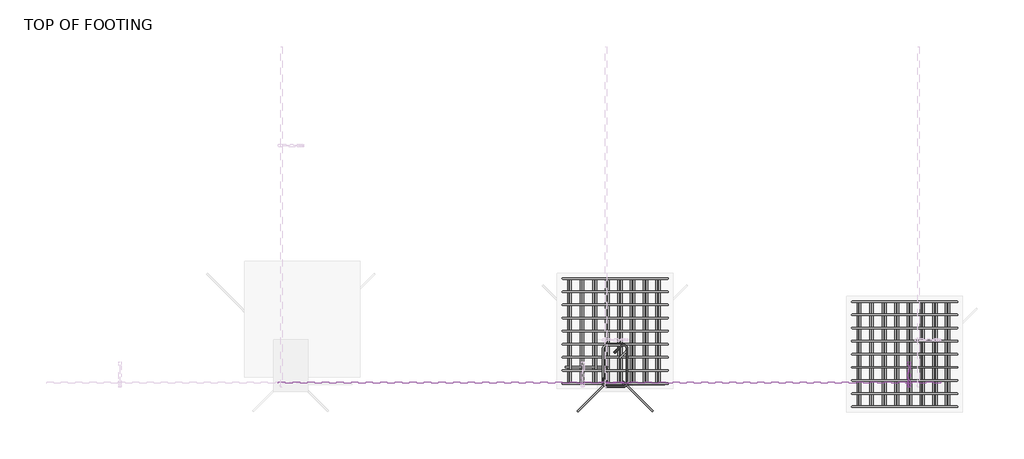
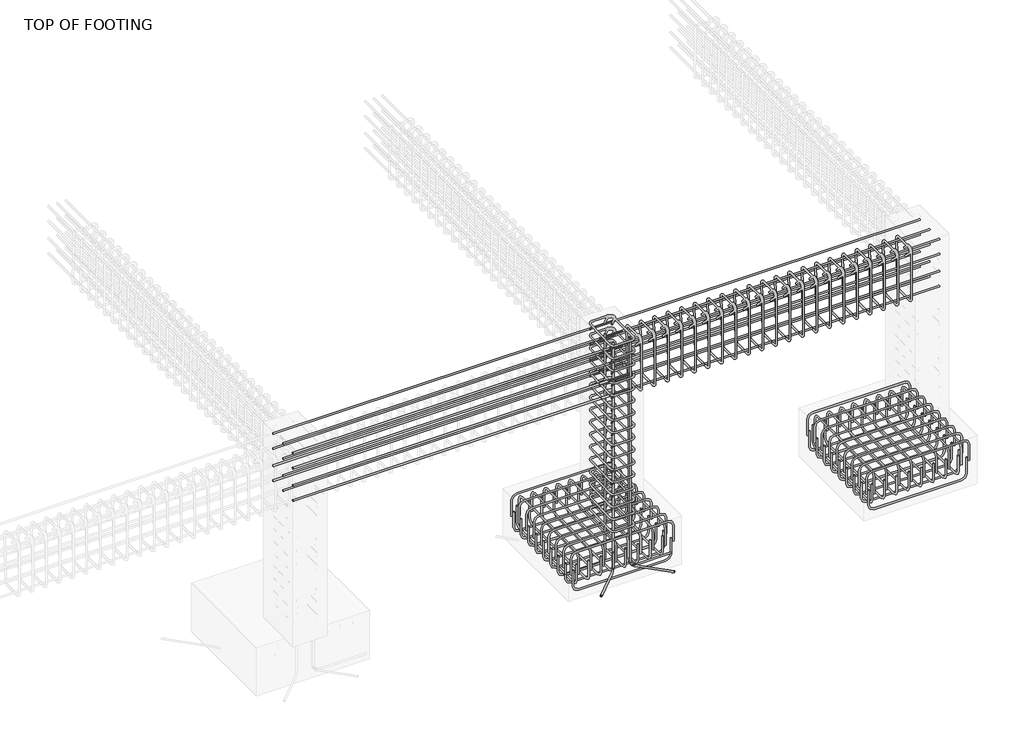
# One storey, part 3 of 14: 22 reinforcing bars.
"""IFC4 building model written with IfcOpenShell, lengths in millimetres."""

from ifc_helpers import new_model, si_unit, point, frame, origin, place, context, project, spatial, polyline, circle_curve, trimmed, segment, composite_curve, source, transform, mapped, element, save
from ifc_brep_helpers import swept_disk

model = new_model("IFC4")

# Units and contexts
model_context = context("Model", 3, world=origin())
ifc_project = project(units=[si_unit("LENGTHUNIT", "METRE", prefix="MILLI")], contexts=[model_context])

# Site, building, storey
site = spatial("IfcSite", under=ifc_project)
building = spatial("IfcBuilding", under=site)
storey = spatial("IfcBuildingStorey", under=building, Name="TOP OF FOOTING", Elevation=-1828.8)

# Reinforcing bars
placement = place(None, origin())
reinforcing_bar_shape = source(origin(), model_context, "Body", "SolidModel", [
    swept_disk(composite_curve([segment(polyline([(4972.542187, 217.7803241, -2035.6107622), (4972.542187, 217.7803241, -2182.9107622)]), True, "CONTINUOUS"), segment(trimmed(circle_curve(frame((4926.192187, 217.7803241, -2182.9107622), z_axis=(0.0, 1.0, 0.0), x_axis=(46.350000000000364, 0.0, 0.0)), 46.35), [point((4972.542187, 217.7803241, -2182.9107622))], [point((4926.192187, 217.7803241, -2229.2607622))], True, "CARTESIAN"), True, "CONTINUOUS"), segment(polyline([(4926.192187, 217.7803241, -2229.2607622), (4153.5617984, 217.7803241, -2229.2607622)]), True, "CONTINUOUS"), segment(trimmed(circle_curve(frame((4153.5617984, 217.7803241, -2182.9107622), z_axis=(0.0, 1.0, 0.0), x_axis=(0.0, 0.0, -46.34999999999991)), 46.35), [point((4153.5617984, 217.7803241, -2229.2607622))], [point((4107.2117984, 217.7803241, -2182.9107622))], True, "CARTESIAN"), True, "CONTINUOUS"), segment(polyline([(4107.2117984, 217.7803241, -2182.9107622), (4107.2117984, 217.7803241, -2035.6107622)]), True, "CONTINUOUS")], self_intersect=False), 6.35),
])
element("IfcReinforcingBar", 1, at=placement, inside=storey, context=model_context, shape_type="MappedRepresentation", body=[
    mapped(reinforcing_bar_shape, transform((0.0, 0.0, 0.0), x_axis=(1.0, 0.0, 0.0), y_axis=(0.0, 1.0, 0.0), z_axis=(0.0, 0.0, 1.0))),
    mapped(reinforcing_bar_shape, transform((0.0, -113.4125, 0.0), x_axis=(1.0, 0.0, 0.0), y_axis=(0.0, 1.0, 0.0), z_axis=(0.0, 0.0, 1.0))),
    mapped(reinforcing_bar_shape, transform((0.0, -226.825, 0.0), x_axis=(1.0, 0.0, 0.0), y_axis=(0.0, 1.0, 0.0), z_axis=(0.0, 0.0, 1.0))),
    mapped(reinforcing_bar_shape, transform((0.0, -340.2375, 0.0), x_axis=(1.0, 0.0, 0.0), y_axis=(0.0, 1.0, 0.0), z_axis=(0.0, 0.0, 1.0))),
    mapped(reinforcing_bar_shape, transform((0.0, -453.65, 0.0), x_axis=(1.0, 0.0, 0.0), y_axis=(0.0, 1.0, 0.0), z_axis=(0.0, 0.0, 1.0))),
    mapped(reinforcing_bar_shape, transform((0.0, -567.0625, 0.0), x_axis=(1.0, 0.0, 0.0), y_axis=(0.0, 1.0, 0.0), z_axis=(0.0, 0.0, 1.0))),
    mapped(reinforcing_bar_shape, transform((0.0, -680.475, 0.0), x_axis=(1.0, 0.0, 0.0), y_axis=(0.0, 1.0, 0.0), z_axis=(0.0, 0.0, 1.0))),
    mapped(reinforcing_bar_shape, transform((0.0, -793.8875, 0.0), x_axis=(1.0, 0.0, 0.0), y_axis=(0.0, 1.0, 0.0), z_axis=(0.0, 0.0, 1.0))),
    mapped(reinforcing_bar_shape, transform((0.0, -907.3, 0.0), x_axis=(1.0, 0.0, 0.0), y_axis=(0.0, 1.0, 0.0), z_axis=(0.0, 0.0, 1.0))),
])
reinforcing_bar_2_shape = source(origin(), model_context, "Body", "SolidModel", [
    swept_disk(composite_curve([segment(polyline([(4088.9966213, 217.7803241, -2068.991024), (4088.9966213, 217.7803241, -1921.691024)]), True, "CONTINUOUS"), segment(trimmed(circle_curve(frame((4135.3466213, 217.7803241, -1921.691024), z_axis=(0.0, 1.0, 0.0), x_axis=(-46.350000000000364, 0.0, 0.0)), 46.35), [point((4088.9966213, 217.7803241, -1921.691024))], [point((4135.3466213, 217.7803241, -1875.341024))], True, "CARTESIAN"), True, "CONTINUOUS"), segment(polyline([(4135.3466213, 217.7803241, -1875.341024), (4949.9466213, 217.7803241, -1875.341024)]), True, "CONTINUOUS"), segment(trimmed(circle_curve(frame((4949.9466213, 217.7803241, -1921.691024), z_axis=(0.0, 1.0, 0.0), x_axis=(0.0, 0.0, 46.34999999999991)), 46.35), [point((4949.9466213, 217.7803241, -1875.341024))], [point((4996.2966213, 217.7803241, -1921.691024))], True, "CARTESIAN"), True, "CONTINUOUS"), segment(polyline([(4996.2966213, 217.7803241, -1921.691024), (4996.2966213, 217.7803241, -2068.991024)]), True, "CONTINUOUS")], self_intersect=False), 6.35),
])
element("IfcReinforcingBar", 2, at=placement, inside=storey, context=model_context, shape_type="MappedRepresentation", body=[
    mapped(reinforcing_bar_2_shape, transform((0.0, 0.0, 0.0), x_axis=(1.0, 0.0, 0.0), y_axis=(0.0, 1.0, 0.0), z_axis=(0.0, 0.0, 1.0))),
    mapped(reinforcing_bar_2_shape, transform((0.0, -113.4125, 0.0), x_axis=(1.0, 0.0, 0.0), y_axis=(0.0, 1.0, 0.0), z_axis=(0.0, 0.0, 1.0))),
    mapped(reinforcing_bar_2_shape, transform((0.0, -226.825, 0.0), x_axis=(1.0, 0.0, 0.0), y_axis=(0.0, 1.0, 0.0), z_axis=(0.0, 0.0, 1.0))),
    mapped(reinforcing_bar_2_shape, transform((0.0, -340.2375, 0.0), x_axis=(1.0, 0.0, 0.0), y_axis=(0.0, 1.0, 0.0), z_axis=(0.0, 0.0, 1.0))),
    mapped(reinforcing_bar_2_shape, transform((0.0, -453.65, 0.0), x_axis=(1.0, 0.0, 0.0), y_axis=(0.0, 1.0, 0.0), z_axis=(0.0, 0.0, 1.0))),
    mapped(reinforcing_bar_2_shape, transform((0.0, -567.0625, 0.0), x_axis=(1.0, 0.0, 0.0), y_axis=(0.0, 1.0, 0.0), z_axis=(0.0, 0.0, 1.0))),
    mapped(reinforcing_bar_2_shape, transform((0.0, -680.475, 0.0), x_axis=(1.0, 0.0, 0.0), y_axis=(0.0, 1.0, 0.0), z_axis=(0.0, 0.0, 1.0))),
    mapped(reinforcing_bar_2_shape, transform((0.0, -793.8875, 0.0), x_axis=(1.0, 0.0, 0.0), y_axis=(0.0, 1.0, 0.0), z_axis=(0.0, 0.0, 1.0))),
    mapped(reinforcing_bar_2_shape, transform((0.0, -907.3, 0.0), x_axis=(1.0, 0.0, 0.0), y_axis=(0.0, 1.0, 0.0), z_axis=(0.0, 0.0, 1.0))),
])
reinforcing_bar_3_shape = source(origin(), model_context, "Body", "SolidModel", [
    swept_disk(composite_curve([segment(polyline([(4926.5067153, 217.7803241, -2085.4684936), (4926.5067153, 217.7803241, -1938.1684936)]), True, "CONTINUOUS"), segment(trimmed(circle_curve(frame((4926.5067153, 171.4303241, -1938.1684936), z_axis=(1.0, 0.0, 0.0), x_axis=(0.0, 46.349999999999994, 0.0)), 46.35), [point((4926.5067153, 217.7803241, -1938.1684936))], [point((4926.5067153, 171.4303241, -1891.8184936))], True, "CARTESIAN"), True, "CONTINUOUS"), segment(polyline([(4926.5067153, 171.4303241, -1891.8184936), (4926.5067153, -643.1696759, -1891.8184936)]), True, "CONTINUOUS"), segment(trimmed(circle_curve(frame((4926.5067153, -643.1696759, -1938.1684936), z_axis=(1.0, 0.0, 0.0), x_axis=(0.0, 0.0, 46.34999999999991)), 46.35), [point((4926.5067153, -643.1696759, -1891.8184936))], [point((4926.5067153, -689.5196759, -1938.1684936))], True, "CARTESIAN"), True, "CONTINUOUS"), segment(polyline([(4926.5067153, -689.5196759, -1938.1684936), (4926.5067153, -689.5196759, -2085.4684936)]), True, "CONTINUOUS")], self_intersect=False), 6.35),
])
element("IfcReinforcingBar", 3, at=placement, inside=storey, context=model_context, shape_type="MappedRepresentation", body=[
    mapped(reinforcing_bar_3_shape, transform((0.0, 0.0, 0.0), x_axis=(1.0, 0.0, 0.0), y_axis=(0.0, 1.0, 0.0), z_axis=(0.0, 0.0, 1.0))),
    mapped(reinforcing_bar_3_shape, transform((-110.0713853, 0.0, 0.0), x_axis=(1.0, 0.0, 0.0), y_axis=(0.0, 1.0, 0.0), z_axis=(0.0, 0.0, 1.0))),
    mapped(reinforcing_bar_3_shape, transform((-220.1427706, 0.0, 0.0), x_axis=(1.0, 0.0, 0.0), y_axis=(0.0, 1.0, 0.0), z_axis=(0.0, 0.0, 1.0))),
    mapped(reinforcing_bar_3_shape, transform((-330.2141558, 0.0, 0.0), x_axis=(1.0, 0.0, 0.0), y_axis=(0.0, 1.0, 0.0), z_axis=(0.0, 0.0, 1.0))),
    mapped(reinforcing_bar_3_shape, transform((-440.2855411, 0.0, 0.0), x_axis=(1.0, 0.0, 0.0), y_axis=(0.0, 1.0, 0.0), z_axis=(0.0, 0.0, 1.0))),
    mapped(reinforcing_bar_3_shape, transform((-550.3569264, 0.0, 0.0), x_axis=(1.0, 0.0, 0.0), y_axis=(0.0, 1.0, 0.0), z_axis=(0.0, 0.0, 1.0))),
    mapped(reinforcing_bar_3_shape, transform((-660.4283117, 0.0, 0.0), x_axis=(1.0, 0.0, 0.0), y_axis=(0.0, 1.0, 0.0), z_axis=(0.0, 0.0, 1.0))),
    mapped(reinforcing_bar_3_shape, transform((-770.4996969, 0.0, 0.0), x_axis=(1.0, 0.0, 0.0), y_axis=(0.0, 1.0, 0.0), z_axis=(0.0, 0.0, 1.0))),
])
reinforcing_bar_4_shape = source(origin(), model_context, "Body", "SolidModel", [
    swept_disk(composite_curve([segment(polyline([(4137.6466213, 217.7803241, -1990.15), (4137.6466213, 217.7803241, -2137.45)]), True, "CONTINUOUS"), segment(trimmed(circle_curve(frame((4137.6466213, 171.4303241, -2137.45), z_axis=(-1.0, 0.0, 0.0), x_axis=(0.0, 46.349999999999994, 0.0)), 46.35), [point((4137.6466213, 217.7803241, -2137.45))], [point((4137.6466213, 171.4303241, -2183.8))], True, "CARTESIAN"), True, "CONTINUOUS"), segment(polyline([(4137.6466213, 171.4303241, -2183.8), (4137.6466213, -643.1696759, -2183.8)]), True, "CONTINUOUS"), segment(trimmed(circle_curve(frame((4137.6466213, -643.1696759, -2137.45), z_axis=(-1.0, 0.0, 0.0), x_axis=(0.0, 0.0, -46.350000000000364)), 46.35), [point((4137.6466213, -643.1696759, -2183.8))], [point((4137.6466213, -689.5196759, -2137.45))], True, "CARTESIAN"), True, "CONTINUOUS"), segment(polyline([(4137.6466213, -689.5196759, -2137.45), (4137.6466213, -689.5196759, -1990.15)]), True, "CONTINUOUS")], self_intersect=False), 6.35),
])
element("IfcReinforcingBar", 4, at=placement, inside=storey, context=model_context, shape_type="MappedRepresentation", body=[
    mapped(reinforcing_bar_4_shape, transform((0.0, 0.0, 0.0), x_axis=(1.0, 0.0, 0.0), y_axis=(0.0, 1.0, 0.0), z_axis=(0.0, 0.0, 1.0))),
    mapped(reinforcing_bar_4_shape, transform((108.7810905, 0.0, 0.0), x_axis=(1.0, 0.0, 0.0), y_axis=(0.0, 1.0, 0.0), z_axis=(0.0, 0.0, 1.0))),
    mapped(reinforcing_bar_4_shape, transform((217.5621811, 0.0, 0.0), x_axis=(1.0, 0.0, 0.0), y_axis=(0.0, 1.0, 0.0), z_axis=(0.0, 0.0, 1.0))),
    mapped(reinforcing_bar_4_shape, transform((326.3432716, 0.0, 0.0), x_axis=(1.0, 0.0, 0.0), y_axis=(0.0, 1.0, 0.0), z_axis=(0.0, 0.0, 1.0))),
    mapped(reinforcing_bar_4_shape, transform((435.1243621, 0.0, 0.0), x_axis=(1.0, 0.0, 0.0), y_axis=(0.0, 1.0, 0.0), z_axis=(0.0, 0.0, 1.0))),
    mapped(reinforcing_bar_4_shape, transform((543.9054526, 0.0, 0.0), x_axis=(1.0, 0.0, 0.0), y_axis=(0.0, 1.0, 0.0), z_axis=(0.0, 0.0, 1.0))),
    mapped(reinforcing_bar_4_shape, transform((652.6865432, 0.0, 0.0), x_axis=(1.0, 0.0, 0.0), y_axis=(0.0, 1.0, 0.0), z_axis=(0.0, 0.0, 1.0))),
    mapped(reinforcing_bar_4_shape, transform((761.4676337, 0.0, 0.0), x_axis=(1.0, 0.0, 0.0), y_axis=(0.0, 1.0, 0.0), z_axis=(0.0, 0.0, 1.0))),
])
reinforcing_bar_5_shape = source(origin(), model_context, "Body", "SolidModel", [
    swept_disk(composite_curve([segment(polyline([(2472.542187, 417.7803241, -2035.6107622), (2472.542187, 417.7803241, -2182.9107622)]), True, "CONTINUOUS"), segment(trimmed(circle_curve(frame((2426.192187, 417.7803241, -2182.9107622), z_axis=(0.0, 1.0, 0.0), x_axis=(46.34999999999991, 0.0, 0.0)), 46.35), [point((2472.542187, 417.7803241, -2182.9107622))], [point((2426.192187, 417.7803241, -2229.2607622))], True, "CARTESIAN"), True, "CONTINUOUS"), segment(polyline([(2426.192187, 417.7803241, -2229.2607622), (1653.5617984, 417.7803241, -2229.2607622)]), True, "CONTINUOUS"), segment(trimmed(circle_curve(frame((1653.5617984, 417.7803241, -2182.9107622), z_axis=(0.0, 1.0, 0.0), x_axis=(0.0, 0.0, -46.34999999999991)), 46.35), [point((1653.5617984, 417.7803241, -2229.2607622))], [point((1607.2117984, 417.7803241, -2182.9107622))], True, "CARTESIAN"), True, "CONTINUOUS"), segment(polyline([(1607.2117984, 417.7803241, -2182.9107622), (1607.2117984, 417.7803241, -2035.6107622)]), True, "CONTINUOUS")], self_intersect=False), 6.35),
])
element("IfcReinforcingBar", 5, at=placement, inside=storey, context=model_context, shape_type="MappedRepresentation", body=[
    mapped(reinforcing_bar_5_shape, transform((0.0, 0.0, 0.0), x_axis=(1.0, 0.0, 0.0), y_axis=(0.0, 1.0, 0.0), z_axis=(0.0, 0.0, 1.0))),
    mapped(reinforcing_bar_5_shape, transform((0.0, -113.4125, 0.0), x_axis=(1.0, 0.0, 0.0), y_axis=(0.0, 1.0, 0.0), z_axis=(0.0, 0.0, 1.0))),
    mapped(reinforcing_bar_5_shape, transform((0.0, -226.825, 0.0), x_axis=(1.0, 0.0, 0.0), y_axis=(0.0, 1.0, 0.0), z_axis=(0.0, 0.0, 1.0))),
    mapped(reinforcing_bar_5_shape, transform((0.0, -340.2375, 0.0), x_axis=(1.0, 0.0, 0.0), y_axis=(0.0, 1.0, 0.0), z_axis=(0.0, 0.0, 1.0))),
    mapped(reinforcing_bar_5_shape, transform((0.0, -453.65, 0.0), x_axis=(1.0, 0.0, 0.0), y_axis=(0.0, 1.0, 0.0), z_axis=(0.0, 0.0, 1.0))),
    mapped(reinforcing_bar_5_shape, transform((0.0, -567.0625, 0.0), x_axis=(1.0, 0.0, 0.0), y_axis=(0.0, 1.0, 0.0), z_axis=(0.0, 0.0, 1.0))),
    mapped(reinforcing_bar_5_shape, transform((0.0, -680.475, 0.0), x_axis=(1.0, 0.0, 0.0), y_axis=(0.0, 1.0, 0.0), z_axis=(0.0, 0.0, 1.0))),
    mapped(reinforcing_bar_5_shape, transform((0.0, -793.8875, 0.0), x_axis=(1.0, 0.0, 0.0), y_axis=(0.0, 1.0, 0.0), z_axis=(0.0, 0.0, 1.0))),
    mapped(reinforcing_bar_5_shape, transform((0.0, -907.3, 0.0), x_axis=(1.0, 0.0, 0.0), y_axis=(0.0, 1.0, 0.0), z_axis=(0.0, 0.0, 1.0))),
])
reinforcing_bar_6_shape = source(origin(), model_context, "Body", "SolidModel", [
    swept_disk(composite_curve([segment(polyline([(1588.9966213, 417.7803241, -2068.991024), (1588.9966213, 417.7803241, -1921.691024)]), True, "CONTINUOUS"), segment(trimmed(circle_curve(frame((1635.3466213, 417.7803241, -1921.691024), z_axis=(0.0, 1.0, 0.0), x_axis=(-46.34999999999991, 0.0, 0.0)), 46.35), [point((1588.9966213, 417.7803241, -1921.691024))], [point((1635.3466213, 417.7803241, -1875.341024))], True, "CARTESIAN"), True, "CONTINUOUS"), segment(polyline([(1635.3466213, 417.7803241, -1875.341024), (2449.9466213, 417.7803241, -1875.341024)]), True, "CONTINUOUS"), segment(trimmed(circle_curve(frame((2449.9466213, 417.7803241, -1921.691024), z_axis=(0.0, 1.0, 0.0), x_axis=(0.0, 0.0, 46.34999999999991)), 46.35), [point((2449.9466213, 417.7803241, -1875.341024))], [point((2496.2966213, 417.7803241, -1921.691024))], True, "CARTESIAN"), True, "CONTINUOUS"), segment(polyline([(2496.2966213, 417.7803241, -1921.691024), (2496.2966213, 417.7803241, -2068.991024)]), True, "CONTINUOUS")], self_intersect=False), 6.35),
])
element("IfcReinforcingBar", 6, at=placement, inside=storey, context=model_context, shape_type="MappedRepresentation", body=[
    mapped(reinforcing_bar_6_shape, transform((0.0, 0.0, 0.0), x_axis=(1.0, 0.0, 0.0), y_axis=(0.0, 1.0, 0.0), z_axis=(0.0, 0.0, 1.0))),
    mapped(reinforcing_bar_6_shape, transform((0.0, -113.4125, 0.0), x_axis=(1.0, 0.0, 0.0), y_axis=(0.0, 1.0, 0.0), z_axis=(0.0, 0.0, 1.0))),
    mapped(reinforcing_bar_6_shape, transform((0.0, -226.825, 0.0), x_axis=(1.0, 0.0, 0.0), y_axis=(0.0, 1.0, 0.0), z_axis=(0.0, 0.0, 1.0))),
    mapped(reinforcing_bar_6_shape, transform((0.0, -340.2375, 0.0), x_axis=(1.0, 0.0, 0.0), y_axis=(0.0, 1.0, 0.0), z_axis=(0.0, 0.0, 1.0))),
    mapped(reinforcing_bar_6_shape, transform((0.0, -453.65, 0.0), x_axis=(1.0, 0.0, 0.0), y_axis=(0.0, 1.0, 0.0), z_axis=(0.0, 0.0, 1.0))),
    mapped(reinforcing_bar_6_shape, transform((0.0, -567.0625, 0.0), x_axis=(1.0, 0.0, 0.0), y_axis=(0.0, 1.0, 0.0), z_axis=(0.0, 0.0, 1.0))),
    mapped(reinforcing_bar_6_shape, transform((0.0, -680.475, 0.0), x_axis=(1.0, 0.0, 0.0), y_axis=(0.0, 1.0, 0.0), z_axis=(0.0, 0.0, 1.0))),
    mapped(reinforcing_bar_6_shape, transform((0.0, -793.8875, 0.0), x_axis=(1.0, 0.0, 0.0), y_axis=(0.0, 1.0, 0.0), z_axis=(0.0, 0.0, 1.0))),
    mapped(reinforcing_bar_6_shape, transform((0.0, -907.3, 0.0), x_axis=(1.0, 0.0, 0.0), y_axis=(0.0, 1.0, 0.0), z_axis=(0.0, 0.0, 1.0))),
])
reinforcing_bar_7_shape = source(origin(), model_context, "Body", "SolidModel", [
    swept_disk(composite_curve([segment(polyline([(2426.5067153, 417.7803241, -2085.4684936), (2426.5067153, 417.7803241, -1938.1684936)]), True, "CONTINUOUS"), segment(trimmed(circle_curve(frame((2426.5067153, 371.4303241, -1938.1684936), z_axis=(1.0, 0.0, 0.0), x_axis=(0.0, 46.349999999999966, 0.0)), 46.35), [point((2426.5067153, 417.7803241, -1938.1684936))], [point((2426.5067153, 371.4303241, -1891.8184936))], True, "CARTESIAN"), True, "CONTINUOUS"), segment(polyline([(2426.5067153, 371.4303241, -1891.8184936), (2426.5067153, -443.1696759, -1891.8184936)]), True, "CONTINUOUS"), segment(trimmed(circle_curve(frame((2426.5067153, -443.1696759, -1938.1684936), z_axis=(1.0, 0.0, 0.0), x_axis=(0.0, 0.0, 46.34999999999991)), 46.35), [point((2426.5067153, -443.1696759, -1891.8184936))], [point((2426.5067153, -489.5196759, -1938.1684936))], True, "CARTESIAN"), True, "CONTINUOUS"), segment(polyline([(2426.5067153, -489.5196759, -1938.1684936), (2426.5067153, -489.5196759, -2085.4684936)]), True, "CONTINUOUS")], self_intersect=False), 6.35),
])
element("IfcReinforcingBar", 7, at=placement, inside=storey, context=model_context, shape_type="MappedRepresentation", body=[
    mapped(reinforcing_bar_7_shape, transform((0.0, 0.0, 0.0), x_axis=(1.0, 0.0, 0.0), y_axis=(0.0, 1.0, 0.0), z_axis=(0.0, 0.0, 1.0))),
    mapped(reinforcing_bar_7_shape, transform((-110.0713853, 0.0, 0.0), x_axis=(1.0, 0.0, 0.0), y_axis=(0.0, 1.0, 0.0), z_axis=(0.0, 0.0, 1.0))),
    mapped(reinforcing_bar_7_shape, transform((-220.1427706, 0.0, 0.0), x_axis=(1.0, 0.0, 0.0), y_axis=(0.0, 1.0, 0.0), z_axis=(0.0, 0.0, 1.0))),
    mapped(reinforcing_bar_7_shape, transform((-330.2141558, 0.0, 0.0), x_axis=(1.0, 0.0, 0.0), y_axis=(0.0, 1.0, 0.0), z_axis=(0.0, 0.0, 1.0))),
    mapped(reinforcing_bar_7_shape, transform((-440.2855411, 0.0, 0.0), x_axis=(1.0, 0.0, 0.0), y_axis=(0.0, 1.0, 0.0), z_axis=(0.0, 0.0, 1.0))),
    mapped(reinforcing_bar_7_shape, transform((-550.3569264, 0.0, 0.0), x_axis=(1.0, 0.0, 0.0), y_axis=(0.0, 1.0, 0.0), z_axis=(0.0, 0.0, 1.0))),
    mapped(reinforcing_bar_7_shape, transform((-660.4283117, 0.0, 0.0), x_axis=(1.0, 0.0, 0.0), y_axis=(0.0, 1.0, 0.0), z_axis=(0.0, 0.0, 1.0))),
    mapped(reinforcing_bar_7_shape, transform((-770.4996969, 0.0, 0.0), x_axis=(1.0, 0.0, 0.0), y_axis=(0.0, 1.0, 0.0), z_axis=(0.0, 0.0, 1.0))),
])
reinforcing_bar_8_shape = source(origin(), model_context, "Body", "SolidModel", [
    swept_disk(composite_curve([segment(polyline([(1637.6466213, 417.7803241, -1990.15), (1637.6466213, 417.7803241, -2137.45)]), True, "CONTINUOUS"), segment(trimmed(circle_curve(frame((1637.6466213, 371.4303241, -2137.45), z_axis=(-1.0, 0.0, 0.0), x_axis=(0.0, 46.349999999999966, 0.0)), 46.35), [point((1637.6466213, 417.7803241, -2137.45))], [point((1637.6466213, 371.4303241, -2183.8))], True, "CARTESIAN"), True, "CONTINUOUS"), segment(polyline([(1637.6466213, 371.4303241, -2183.8), (1637.6466213, -443.1696759, -2183.8)]), True, "CONTINUOUS"), segment(trimmed(circle_curve(frame((1637.6466213, -443.1696759, -2137.45), z_axis=(-1.0, 0.0, 0.0), x_axis=(0.0, 0.0, -46.350000000000364)), 46.35), [point((1637.6466213, -443.1696759, -2183.8))], [point((1637.6466213, -489.5196759, -2137.45))], True, "CARTESIAN"), True, "CONTINUOUS"), segment(polyline([(1637.6466213, -489.5196759, -2137.45), (1637.6466213, -489.5196759, -1990.15)]), True, "CONTINUOUS")], self_intersect=False), 6.35),
])
element("IfcReinforcingBar", 8, at=placement, inside=storey, context=model_context, shape_type="MappedRepresentation", body=[
    mapped(reinforcing_bar_8_shape, transform((0.0, 0.0, 0.0), x_axis=(1.0, 0.0, 0.0), y_axis=(0.0, 1.0, 0.0), z_axis=(0.0, 0.0, 1.0))),
    mapped(reinforcing_bar_8_shape, transform((108.7810905, 0.0, 0.0), x_axis=(1.0, 0.0, 0.0), y_axis=(0.0, 1.0, 0.0), z_axis=(0.0, 0.0, 1.0))),
    mapped(reinforcing_bar_8_shape, transform((217.5621811, 0.0, 0.0), x_axis=(1.0, 0.0, 0.0), y_axis=(0.0, 1.0, 0.0), z_axis=(0.0, 0.0, 1.0))),
    mapped(reinforcing_bar_8_shape, transform((326.3432716, 0.0, 0.0), x_axis=(1.0, 0.0, 0.0), y_axis=(0.0, 1.0, 0.0), z_axis=(0.0, 0.0, 1.0))),
    mapped(reinforcing_bar_8_shape, transform((435.1243621, 0.0, 0.0), x_axis=(1.0, 0.0, 0.0), y_axis=(0.0, 1.0, 0.0), z_axis=(0.0, 0.0, 1.0))),
    mapped(reinforcing_bar_8_shape, transform((543.9054526, 0.0, 0.0), x_axis=(1.0, 0.0, 0.0), y_axis=(0.0, 1.0, 0.0), z_axis=(0.0, 0.0, 1.0))),
    mapped(reinforcing_bar_8_shape, transform((652.6865432, 0.0, 0.0), x_axis=(1.0, 0.0, 0.0), y_axis=(0.0, 1.0, 0.0), z_axis=(0.0, 0.0, 1.0))),
    mapped(reinforcing_bar_8_shape, transform((761.4676337, 0.0, 0.0), x_axis=(1.0, 0.0, 0.0), y_axis=(0.0, 1.0, 0.0), z_axis=(0.0, 0.0, 1.0))),
])
reinforcing_bar_9_shape = source(origin(), model_context, "Body", "SolidModel", [
    swept_disk(composite_curve([segment(polyline([(2037.0352608, -222.1454413, -46.35), (2092.7788237, -166.4018783, -46.35)]), True, "CONTINUOUS"), segment(trimmed(circle_curve(frame((2114.9466213, -188.5696759, -46.35), z_axis=(0.0, 0.0, -1.0), x_axis=(-22.167797600000085, 22.1677976, 0.0)), 31.35), [point((2092.7788237, -166.4018783, -46.35))], [point((2146.2966213, -188.5696759, -46.35))], True, "CARTESIAN"), True, "CONTINUOUS"), segment(polyline([(2146.2966213, -188.5696759, -46.35), (2146.2966213, -483.1696759, -46.35)]), True, "CONTINUOUS"), segment(trimmed(circle_curve(frame((2114.9466213, -483.1696759, -46.35), z_axis=(0.0, 0.0, -1.0), x_axis=(31.34999999999991, 0.0, 0.0)), 31.35), [point((2146.2966213, -483.1696759, -46.35))], [point((2114.9466213, -514.5196759, -46.35))], True, "CARTESIAN"), True, "CONTINUOUS"), segment(polyline([(2114.9466213, -514.5196759, -46.35), (1970.3466213, -514.5196759, -46.35)]), True, "CONTINUOUS"), segment(trimmed(circle_curve(frame((1970.3466213, -483.189461, -45.2363875), z_axis=(0.0, 0.03552192833448213, -0.9993688971583016), x_axis=(0.0, -31.330214900000044, -1.1136125000000021)), 31.35), [point((1970.3466213, -514.5196759, -46.35))], [point((1938.9966213, -483.189461, -45.2363875))], True, "CARTESIAN"), True, "CONTINUOUS"), segment(polyline([(1938.9966213, -483.189461, -45.2363875), (1938.9966213, -188.5498908, -34.7636125)]), True, "CONTINUOUS"), segment(trimmed(circle_curve(frame((1970.3466213, -188.5498908, -34.7636125), z_axis=(0.0, 0.03552192833448213, -0.9993688971583016), x_axis=(-31.34999999999991, 0.0, 0.0)), 31.35), [point((1938.9966213, -188.5498908, -34.7636125))], [point((1970.3466213, -157.2196759, -33.65))], True, "CARTESIAN"), True, "CONTINUOUS"), segment(polyline([(1970.3466213, -157.2196759, -33.65), (2114.9466213, -157.2196759, -33.65)]), True, "CONTINUOUS"), segment(trimmed(circle_curve(frame((2114.9466213, -188.5696759, -33.65), z_axis=(0.0, 0.0, -1.0), x_axis=(0.0, 31.349999999999994, 0.0)), 31.35), [point((2114.9466213, -157.2196759, -33.65))], [point((2137.1144189, -210.7374735, -33.65))], True, "CARTESIAN"), True, "CONTINUOUS"), segment(polyline([(2137.1144189, -210.7374735, -33.65), (2081.3708559, -266.4810364, -33.65)]), True, "CONTINUOUS")], self_intersect=False), 6.35),
])
element("IfcReinforcingBar", 9, at=placement, inside=storey, context=model_context, shape_type="MappedRepresentation", body=[
    mapped(reinforcing_bar_9_shape, transform((0.0, 0.0, 0.0), x_axis=(1.0, 0.0, 0.0), y_axis=(0.0, 1.0, 0.0), z_axis=(0.0, 0.0, 1.0))),
    mapped(reinforcing_bar_9_shape, transform((0.0, 0.0, -115.74), x_axis=(1.0, 0.0, 0.0), y_axis=(0.0, 1.0, 0.0), z_axis=(0.0, 0.0, 1.0))),
    mapped(reinforcing_bar_9_shape, transform((0.0, 0.0, -231.48), x_axis=(1.0, 0.0, 0.0), y_axis=(0.0, 1.0, 0.0), z_axis=(0.0, 0.0, 1.0))),
    mapped(reinforcing_bar_9_shape, transform((0.0, 0.0, -347.22), x_axis=(1.0, 0.0, 0.0), y_axis=(0.0, 1.0, 0.0), z_axis=(0.0, 0.0, 1.0))),
    mapped(reinforcing_bar_9_shape, transform((0.0, 0.0, -462.96), x_axis=(1.0, 0.0, 0.0), y_axis=(0.0, 1.0, 0.0), z_axis=(0.0, 0.0, 1.0))),
    mapped(reinforcing_bar_9_shape, transform((0.0, 0.0, -578.7), x_axis=(1.0, 0.0, 0.0), y_axis=(0.0, 1.0, 0.0), z_axis=(0.0, 0.0, 1.0))),
    mapped(reinforcing_bar_9_shape, transform((0.0, 0.0, -694.44), x_axis=(1.0, 0.0, 0.0), y_axis=(0.0, 1.0, 0.0), z_axis=(0.0, 0.0, 1.0))),
    mapped(reinforcing_bar_9_shape, transform((0.0, 0.0, -810.18), x_axis=(1.0, 0.0, 0.0), y_axis=(0.0, 1.0, 0.0), z_axis=(0.0, 0.0, 1.0))),
    mapped(reinforcing_bar_9_shape, transform((0.0, 0.0, -925.92), x_axis=(1.0, 0.0, 0.0), y_axis=(0.0, 1.0, 0.0), z_axis=(0.0, 0.0, 1.0))),
    mapped(reinforcing_bar_9_shape, transform((0.0, 0.0, -1041.66), x_axis=(1.0, 0.0, 0.0), y_axis=(0.0, 1.0, 0.0), z_axis=(0.0, 0.0, 1.0))),
    mapped(reinforcing_bar_9_shape, transform((0.0, 0.0, -1157.4), x_axis=(1.0, 0.0, 0.0), y_axis=(0.0, 1.0, 0.0), z_axis=(0.0, 0.0, 1.0))),
    mapped(reinforcing_bar_9_shape, transform((0.0, 0.0, -1273.14), x_axis=(1.0, 0.0, 0.0), y_axis=(0.0, 1.0, 0.0), z_axis=(0.0, 0.0, 1.0))),
    mapped(reinforcing_bar_9_shape, transform((0.0, 0.0, -1388.88), x_axis=(1.0, 0.0, 0.0), y_axis=(0.0, 1.0, 0.0), z_axis=(0.0, 0.0, 1.0))),
    mapped(reinforcing_bar_9_shape, transform((0.0, 0.0, -1504.62), x_axis=(1.0, 0.0, 0.0), y_axis=(0.0, 1.0, 0.0), z_axis=(0.0, 0.0, 1.0))),
    mapped(reinforcing_bar_9_shape, transform((0.0, 0.0, -1620.36), x_axis=(1.0, 0.0, 0.0), y_axis=(0.0, 1.0, 0.0), z_axis=(0.0, 0.0, 1.0))),
    mapped(reinforcing_bar_9_shape, transform((0.0, 0.0, -1736.1), x_axis=(1.0, 0.0, 0.0), y_axis=(0.0, 1.0, 0.0), z_axis=(0.0, 0.0, 1.0))),
])
element("IfcReinforcingBar", 10, at=placement, inside=storey, context=model_context, shape_type="SolidModel", body=[
    swept_disk(composite_curve([segment(polyline([(2113.2979629, -495.9487744, -40.0), (2113.2979629, -495.9487744, -2122.4113862)]), True, "CONTINUOUS"), segment(trimmed(circle_curve(frame((2159.6479629, -495.9487744, -2122.4113862), z_axis=(0.0, -1.0, 0.0), x_axis=(-46.34999999999991, 0.0, 0.0)), 46.35), [point((2113.2979629, -495.9487744, -2122.4113862))], [point((2159.6479629, -495.9487744, -2168.7613862))], True, "CARTESIAN"), True, "CONTINUOUS"), segment(polyline([(2159.6479629, -495.9487744, -2168.7613862), (2471.7593977, -495.9487744, -2168.7613862)]), True, "CONTINUOUS")], self_intersect=False), 6.35),
])
element("IfcReinforcingBar", 11, at=placement, inside=storey, context=model_context, shape_type="SolidModel", body=[
    swept_disk(composite_curve([segment(polyline([(2113.2979629, -475.9487744, -40.0), (2113.2979629, -475.9487744, -2122.4113862)]), True, "CONTINUOUS"), segment(trimmed(circle_curve(frame((2146.0723622, -508.7231737, -2122.4113862), z_axis=(-0.7071067811865441, -0.707106781186551, 0.0), x_axis=(-32.774399299999914, 32.77439930000003, 0.0)), 46.35), [point((2113.2979629, -475.9487744, -2122.4113862))], [point((2146.0723622, -508.7231737, -2168.7613862))], True, "CARTESIAN"), True, "CONTINUOUS"), segment(polyline([(2146.0723622, -508.7231737, -2168.7613862), (2366.7684742, -729.4192858, -2168.7613862)]), True, "CONTINUOUS")], self_intersect=False), 6.35),
])
element("IfcReinforcingBar", 12, at=placement, inside=storey, context=model_context, shape_type="SolidModel", body=[
    swept_disk(composite_curve([segment(polyline([(1971.9952797, -475.9487744, -40.0), (1971.9952797, -475.9487744, -2122.4113862)]), True, "CONTINUOUS"), segment(trimmed(circle_curve(frame((1939.2208804, -508.7231737, -2122.4113862), z_axis=(-0.7071067811865341, 0.707106781186561, 0.0), x_axis=(32.77439930000014, 32.77439930000003, 0.0)), 46.35), [point((1971.9952797, -475.9487744, -2122.4113862))], [point((1939.2208804, -508.7231737, -2168.7613862))], True, "CARTESIAN"), True, "CONTINUOUS"), segment(polyline([(1939.2208804, -508.7231737, -2168.7613862), (1718.5247684, -729.4192858, -2168.7613862)]), True, "CONTINUOUS")], self_intersect=False), 6.35),
])
element("IfcReinforcingBar", 13, at=placement, inside=storey, context=model_context, shape_type="SolidModel", body=[
    swept_disk(composite_curve([segment(polyline([(1971.9952797, -345.9487744, -40.0), (1971.9952797, -345.9487744, -2122.4113862)]), True, "CONTINUOUS"), segment(trimmed(circle_curve(frame((1925.6452797, -345.9487744, -2122.4113862), z_axis=(0.0, 1.0, 0.0), x_axis=(46.350000000000136, 0.0, 0.0)), 46.35), [point((1971.9952797, -345.9487744, -2122.4113862))], [point((1925.6452797, -345.9487744, -2168.7613862))], True, "CARTESIAN"), True, "CONTINUOUS"), segment(polyline([(1925.6452797, -345.9487744, -2168.7613862), (1613.5338449, -345.9487744, -2168.7613862)]), True, "CONTINUOUS")], self_intersect=False), 6.35),
])
reinforcing_bar_10_shape = source(origin(), model_context, "Body", "SolidModel", [
    swept_disk(composite_curve([segment(polyline([(-867.3533787, -181.1234225, -77.7), (2152.6466213, -181.1234225, -77.7)]), True, "CONTINUOUS")], self_intersect=False), 6.35),
])
element("IfcReinforcingBar", 14, at=placement, inside=storey, context=model_context, shape_type="MappedRepresentation", body=[
    mapped(reinforcing_bar_10_shape, transform((0.0, 0.0, 0.0), x_axis=(1.0, 0.0, 0.0), y_axis=(0.0, 1.0, 0.0), z_axis=(0.0, 0.0, 1.0))),
    mapped(reinforcing_bar_10_shape, transform((0.0, -151.0102945, 0.0), x_axis=(1.0, 0.0, 0.0), y_axis=(0.0, 1.0, 0.0), z_axis=(0.0, 0.0, 1.0))),
    mapped(reinforcing_bar_10_shape, transform((0.0, -302.0205889, 0.0), x_axis=(1.0, 0.0, 0.0), y_axis=(0.0, 1.0, 0.0), z_axis=(0.0, 0.0, 1.0))),
])
reinforcing_bar_11_shape = source(origin(), model_context, "Body", "SolidModel", [
    swept_disk(composite_curve([segment(polyline([(-867.3533787, -181.1234225, -517.7), (2152.6466213, -181.1234225, -517.7)]), True, "CONTINUOUS")], self_intersect=False), 6.35),
])
element("IfcReinforcingBar", 15, at=placement, inside=storey, context=model_context, shape_type="MappedRepresentation", body=[
    mapped(reinforcing_bar_11_shape, transform((0.0, 0.0, 0.0), x_axis=(1.0, 0.0, 0.0), y_axis=(0.0, 1.0, 0.0), z_axis=(0.0, 0.0, 1.0))),
    mapped(reinforcing_bar_11_shape, transform((0.0, -151.0102945, 0.0), x_axis=(1.0, 0.0, 0.0), y_axis=(0.0, 1.0, 0.0), z_axis=(0.0, 0.0, 1.0))),
    mapped(reinforcing_bar_11_shape, transform((0.0, -302.0205889, 0.0), x_axis=(1.0, 0.0, 0.0), y_axis=(0.0, 1.0, 0.0), z_axis=(0.0, 0.0, 1.0))),
])
reinforcing_bar_12_shape = source(origin(), model_context, "Body", "SolidModel", [
    swept_disk(composite_curve([segment(polyline([(-867.3533787, -181.1234225, -377.7), (2152.6466213, -181.1234225, -377.7)]), True, "CONTINUOUS")], self_intersect=False), 6.35),
])
element("IfcReinforcingBar", 16, at=placement, inside=storey, context=model_context, shape_type="MappedRepresentation", body=[
    mapped(reinforcing_bar_12_shape, transform((0.0, 0.0, 0.0), x_axis=(1.0, 0.0, 0.0), y_axis=(0.0, 1.0, 0.0), z_axis=(0.0, 0.0, 1.0))),
    mapped(reinforcing_bar_12_shape, transform((0.0, -151.0102945, 0.0), x_axis=(1.0, 0.0, 0.0), y_axis=(0.0, 1.0, 0.0), z_axis=(0.0, 0.0, 1.0))),
    mapped(reinforcing_bar_12_shape, transform((0.0, -302.0205889, 0.0), x_axis=(1.0, 0.0, 0.0), y_axis=(0.0, 1.0, 0.0), z_axis=(0.0, 0.0, 1.0))),
])
reinforcing_bar_13_shape = source(origin(), model_context, "Body", "SolidModel", [
    swept_disk(composite_curve([segment(polyline([(-867.3533787, -181.1234225, -217.7), (2152.6466213, -181.1234225, -217.7)]), True, "CONTINUOUS")], self_intersect=False), 6.35),
])
element("IfcReinforcingBar", 17, at=placement, inside=storey, context=model_context, shape_type="MappedRepresentation", body=[
    mapped(reinforcing_bar_13_shape, transform((0.0, 0.0, 0.0), x_axis=(1.0, 0.0, 0.0), y_axis=(0.0, 1.0, 0.0), z_axis=(0.0, 0.0, 1.0))),
    mapped(reinforcing_bar_13_shape, transform((0.0, -151.0102945, 0.0), x_axis=(1.0, 0.0, 0.0), y_axis=(0.0, 1.0, 0.0), z_axis=(0.0, 0.0, 1.0))),
    mapped(reinforcing_bar_13_shape, transform((0.0, -302.0205889, 0.0), x_axis=(1.0, 0.0, 0.0), y_axis=(0.0, 1.0, 0.0), z_axis=(0.0, 0.0, 1.0))),
])
reinforcing_bar_14_shape = source(origin(), model_context, "Body", "SolidModel", [
    swept_disk(composite_curve([segment(polyline([(2198.9966213, -405.2583154, -111.2757654), (2198.9966213, -461.0018783, -55.5322024)]), True, "CONTINUOUS"), segment(trimmed(circle_curve(frame((2198.9966213, -483.1696759, -77.7), z_axis=(1.0, 0.0, 0.0), x_axis=(0.0, 22.16779760000003, 22.1677976)), 31.35), [point((2198.9966213, -461.0018783, -55.5322024))], [point((2198.9966213, -514.5196759, -77.7))], True, "CARTESIAN"), True, "CONTINUOUS"), segment(polyline([(2198.9966213, -514.5196759, -77.7), (2198.9966213, -514.5196759, -522.3)]), True, "CONTINUOUS"), segment(trimmed(circle_curve(frame((2198.9966213, -483.1696759, -522.3), z_axis=(1.0, 0.0, 0.0), x_axis=(0.0, -31.350000000000023, 0.0)), 31.35), [point((2198.9966213, -514.5196759, -522.3))], [point((2198.9966213, -483.1696759, -553.65))], True, "CARTESIAN"), True, "CONTINUOUS"), segment(polyline([(2198.9966213, -483.1696759, -553.65), (2198.9966213, -338.5696759, -553.65)]), True, "CONTINUOUS"), segment(trimmed(circle_curve(frame((2198.2120357, -338.5696759, -522.3098193), z_axis=(0.9996867842138424, 0.0, 0.025026655153786322), x_axis=(0.7845855999999003, 0.0, -31.34018070000002)), 31.35), [point((2198.9966213, -338.5696759, -553.65))], [point((2198.2120357, -307.2196759, -522.3098193))], True, "CARTESIAN"), True, "CONTINUOUS"), segment(polyline([(2198.2120357, -307.2196759, -522.3098193), (2187.0812069, -307.2196759, -77.6901807)]), True, "CONTINUOUS"), segment(trimmed(circle_curve(frame((2187.0812069, -338.5696759, -77.6901807), z_axis=(0.9996867842138424, 0.0, 0.025026655153786322), x_axis=(0.0, 31.349999999999966, 0.0)), 31.35), [point((2187.0812069, -307.2196759, -77.6901807))], [point((2186.2966213, -338.5696759, -46.35))], True, "CARTESIAN"), True, "CONTINUOUS"), segment(polyline([(2186.2966213, -338.5696759, -46.35), (2186.2966213, -483.1696759, -46.35)]), True, "CONTINUOUS"), segment(trimmed(circle_curve(frame((2186.2966213, -483.1696759, -77.7), z_axis=(1.0, 0.0, 0.0), x_axis=(0.0, 0.0, 31.35)), 31.35), [point((2186.2966213, -483.1696759, -46.35))], [point((2186.2966213, -505.3374735, -99.8677976))], True, "CARTESIAN"), True, "CONTINUOUS"), segment(polyline([(2186.2966213, -505.3374735, -99.8677976), (2186.2966213, -449.5939106, -155.6113605)]), True, "CONTINUOUS")], self_intersect=False), 6.35),
])
element("IfcReinforcingBar", 18, at=placement, inside=storey, context=model_context, shape_type="MappedRepresentation", body=[
    mapped(reinforcing_bar_14_shape, transform((0.0, 0.0, 0.0), x_axis=(1.0, 0.0, 0.0), y_axis=(0.0, 1.0, 0.0), z_axis=(0.0, 0.0, 1.0))),
    mapped(reinforcing_bar_14_shape, transform((119.365, 0.0, 0.0), x_axis=(1.0, 0.0, 0.0), y_axis=(0.0, 1.0, 0.0), z_axis=(0.0, 0.0, 1.0))),
    mapped(reinforcing_bar_14_shape, transform((238.73, 0.0, 0.0), x_axis=(1.0, 0.0, 0.0), y_axis=(0.0, 1.0, 0.0), z_axis=(0.0, 0.0, 1.0))),
    mapped(reinforcing_bar_14_shape, transform((358.095, 0.0, 0.0), x_axis=(1.0, 0.0, 0.0), y_axis=(0.0, 1.0, 0.0), z_axis=(0.0, 0.0, 1.0))),
    mapped(reinforcing_bar_14_shape, transform((477.46, 0.0, 0.0), x_axis=(1.0, 0.0, 0.0), y_axis=(0.0, 1.0, 0.0), z_axis=(0.0, 0.0, 1.0))),
    mapped(reinforcing_bar_14_shape, transform((596.825, 0.0, 0.0), x_axis=(1.0, 0.0, 0.0), y_axis=(0.0, 1.0, 0.0), z_axis=(0.0, 0.0, 1.0))),
    mapped(reinforcing_bar_14_shape, transform((716.19, 0.0, 0.0), x_axis=(1.0, 0.0, 0.0), y_axis=(0.0, 1.0, 0.0), z_axis=(0.0, 0.0, 1.0))),
    mapped(reinforcing_bar_14_shape, transform((835.555, 0.0, 0.0), x_axis=(1.0, 0.0, 0.0), y_axis=(0.0, 1.0, 0.0), z_axis=(0.0, 0.0, 1.0))),
    mapped(reinforcing_bar_14_shape, transform((954.92, 0.0, 0.0), x_axis=(1.0, 0.0, 0.0), y_axis=(0.0, 1.0, 0.0), z_axis=(0.0, 0.0, 1.0))),
    mapped(reinforcing_bar_14_shape, transform((1074.285, 0.0, 0.0), x_axis=(1.0, 0.0, 0.0), y_axis=(0.0, 1.0, 0.0), z_axis=(0.0, 0.0, 1.0))),
    mapped(reinforcing_bar_14_shape, transform((1193.65, 0.0, 0.0), x_axis=(1.0, 0.0, 0.0), y_axis=(0.0, 1.0, 0.0), z_axis=(0.0, 0.0, 1.0))),
    mapped(reinforcing_bar_14_shape, transform((1313.015, 0.0, 0.0), x_axis=(1.0, 0.0, 0.0), y_axis=(0.0, 1.0, 0.0), z_axis=(0.0, 0.0, 1.0))),
    mapped(reinforcing_bar_14_shape, transform((1432.38, 0.0, 0.0), x_axis=(1.0, 0.0, 0.0), y_axis=(0.0, 1.0, 0.0), z_axis=(0.0, 0.0, 1.0))),
    mapped(reinforcing_bar_14_shape, transform((1551.745, 0.0, 0.0), x_axis=(1.0, 0.0, 0.0), y_axis=(0.0, 1.0, 0.0), z_axis=(0.0, 0.0, 1.0))),
    mapped(reinforcing_bar_14_shape, transform((1671.11, 0.0, 0.0), x_axis=(1.0, 0.0, 0.0), y_axis=(0.0, 1.0, 0.0), z_axis=(0.0, 0.0, 1.0))),
    mapped(reinforcing_bar_14_shape, transform((1790.475, 0.0, 0.0), x_axis=(1.0, 0.0, 0.0), y_axis=(0.0, 1.0, 0.0), z_axis=(0.0, 0.0, 1.0))),
    mapped(reinforcing_bar_14_shape, transform((1909.84, 0.0, 0.0), x_axis=(1.0, 0.0, 0.0), y_axis=(0.0, 1.0, 0.0), z_axis=(0.0, 0.0, 1.0))),
    mapped(reinforcing_bar_14_shape, transform((2029.205, 0.0, 0.0), x_axis=(1.0, 0.0, 0.0), y_axis=(0.0, 1.0, 0.0), z_axis=(0.0, 0.0, 1.0))),
    mapped(reinforcing_bar_14_shape, transform((2148.57, 0.0, 0.0), x_axis=(1.0, 0.0, 0.0), y_axis=(0.0, 1.0, 0.0), z_axis=(0.0, 0.0, 1.0))),
    mapped(reinforcing_bar_14_shape, transform((2267.935, 0.0, 0.0), x_axis=(1.0, 0.0, 0.0), y_axis=(0.0, 1.0, 0.0), z_axis=(0.0, 0.0, 1.0))),
    mapped(reinforcing_bar_14_shape, transform((2387.3, 0.0, 0.0), x_axis=(1.0, 0.0, 0.0), y_axis=(0.0, 1.0, 0.0), z_axis=(0.0, 0.0, 1.0))),
])
reinforcing_bar_15_shape = source(origin(), model_context, "Body", "SolidModel", [
    swept_disk(composite_curve([segment(polyline([(1932.6466213, -181.1234225, -77.7), (4852.6466213, -181.1234225, -77.7)]), True, "CONTINUOUS")], self_intersect=False), 6.35),
])
element("IfcReinforcingBar", 19, at=placement, inside=storey, context=model_context, shape_type="MappedRepresentation", body=[
    mapped(reinforcing_bar_15_shape, transform((0.0, 0.0, 0.0), x_axis=(1.0, 0.0, 0.0), y_axis=(0.0, 1.0, 0.0), z_axis=(0.0, 0.0, 1.0))),
    mapped(reinforcing_bar_15_shape, transform((0.0, -151.0102945, 0.0), x_axis=(1.0, 0.0, 0.0), y_axis=(0.0, 1.0, 0.0), z_axis=(0.0, 0.0, 1.0))),
    mapped(reinforcing_bar_15_shape, transform((0.0, -302.0205889, 0.0), x_axis=(1.0, 0.0, 0.0), y_axis=(0.0, 1.0, 0.0), z_axis=(0.0, 0.0, 1.0))),
])
reinforcing_bar_16_shape = source(origin(), model_context, "Body", "SolidModel", [
    swept_disk(composite_curve([segment(polyline([(1932.6466213, -181.1234225, -517.7), (4852.6466213, -181.1234225, -517.7)]), True, "CONTINUOUS")], self_intersect=False), 6.35),
])
element("IfcReinforcingBar", 20, at=placement, inside=storey, context=model_context, shape_type="MappedRepresentation", body=[
    mapped(reinforcing_bar_16_shape, transform((0.0, 0.0, 0.0), x_axis=(1.0, 0.0, 0.0), y_axis=(0.0, 1.0, 0.0), z_axis=(0.0, 0.0, 1.0))),
    mapped(reinforcing_bar_16_shape, transform((0.0, -151.0102945, 0.0), x_axis=(1.0, 0.0, 0.0), y_axis=(0.0, 1.0, 0.0), z_axis=(0.0, 0.0, 1.0))),
    mapped(reinforcing_bar_16_shape, transform((0.0, -302.0205889, 0.0), x_axis=(1.0, 0.0, 0.0), y_axis=(0.0, 1.0, 0.0), z_axis=(0.0, 0.0, 1.0))),
])
reinforcing_bar_17_shape = source(origin(), model_context, "Body", "SolidModel", [
    swept_disk(composite_curve([segment(polyline([(1932.6466213, -181.1234225, -377.7), (4852.6466213, -181.1234225, -377.7)]), True, "CONTINUOUS")], self_intersect=False), 6.35),
])
element("IfcReinforcingBar", 21, at=placement, inside=storey, context=model_context, shape_type="MappedRepresentation", body=[
    mapped(reinforcing_bar_17_shape, transform((0.0, 0.0, 0.0), x_axis=(1.0, 0.0, 0.0), y_axis=(0.0, 1.0, 0.0), z_axis=(0.0, 0.0, 1.0))),
    mapped(reinforcing_bar_17_shape, transform((0.0, -151.0102945, 0.0), x_axis=(1.0, 0.0, 0.0), y_axis=(0.0, 1.0, 0.0), z_axis=(0.0, 0.0, 1.0))),
    mapped(reinforcing_bar_17_shape, transform((0.0, -302.0205889, 0.0), x_axis=(1.0, 0.0, 0.0), y_axis=(0.0, 1.0, 0.0), z_axis=(0.0, 0.0, 1.0))),
])
reinforcing_bar_18_shape = source(origin(), model_context, "Body", "SolidModel", [
    swept_disk(composite_curve([segment(polyline([(1932.6466213, -181.1234225, -217.7), (4852.6466213, -181.1234225, -217.7)]), True, "CONTINUOUS")], self_intersect=False), 6.35),
])
element("IfcReinforcingBar", 22, at=placement, inside=storey, context=model_context, shape_type="MappedRepresentation", body=[
    mapped(reinforcing_bar_18_shape, transform((0.0, 0.0, 0.0), x_axis=(1.0, 0.0, 0.0), y_axis=(0.0, 1.0, 0.0), z_axis=(0.0, 0.0, 1.0))),
    mapped(reinforcing_bar_18_shape, transform((0.0, -151.0102945, 0.0), x_axis=(1.0, 0.0, 0.0), y_axis=(0.0, 1.0, 0.0), z_axis=(0.0, 0.0, 1.0))),
    mapped(reinforcing_bar_18_shape, transform((0.0, -302.0205889, 0.0), x_axis=(1.0, 0.0, 0.0), y_axis=(0.0, 1.0, 0.0), z_axis=(0.0, 0.0, 1.0))),
])

save(model, "model.ifc")

# Revit data of these elements
# Elements 1, 2, 3, 4, 5, 6, 7, 8, 9, 10, 11, 12, 13, 14, 15, 16, 17, 18, 19, 20, 21, 22 (IfcReinforcingBar)
#   Phase Created = New Construction
